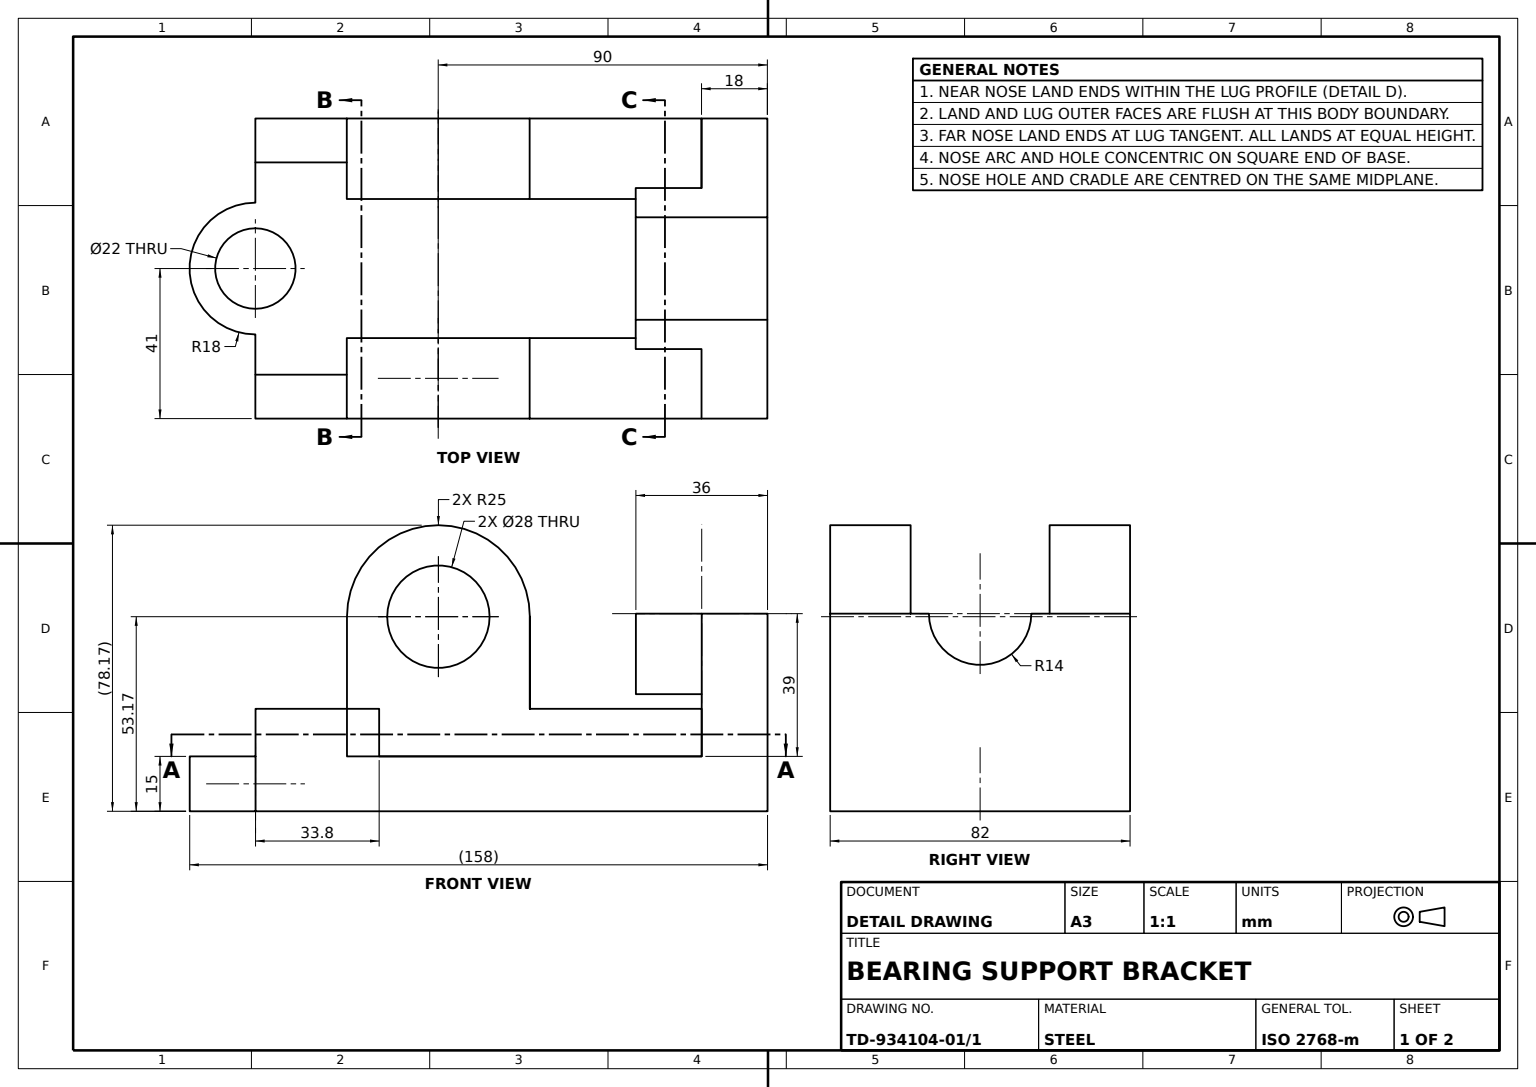
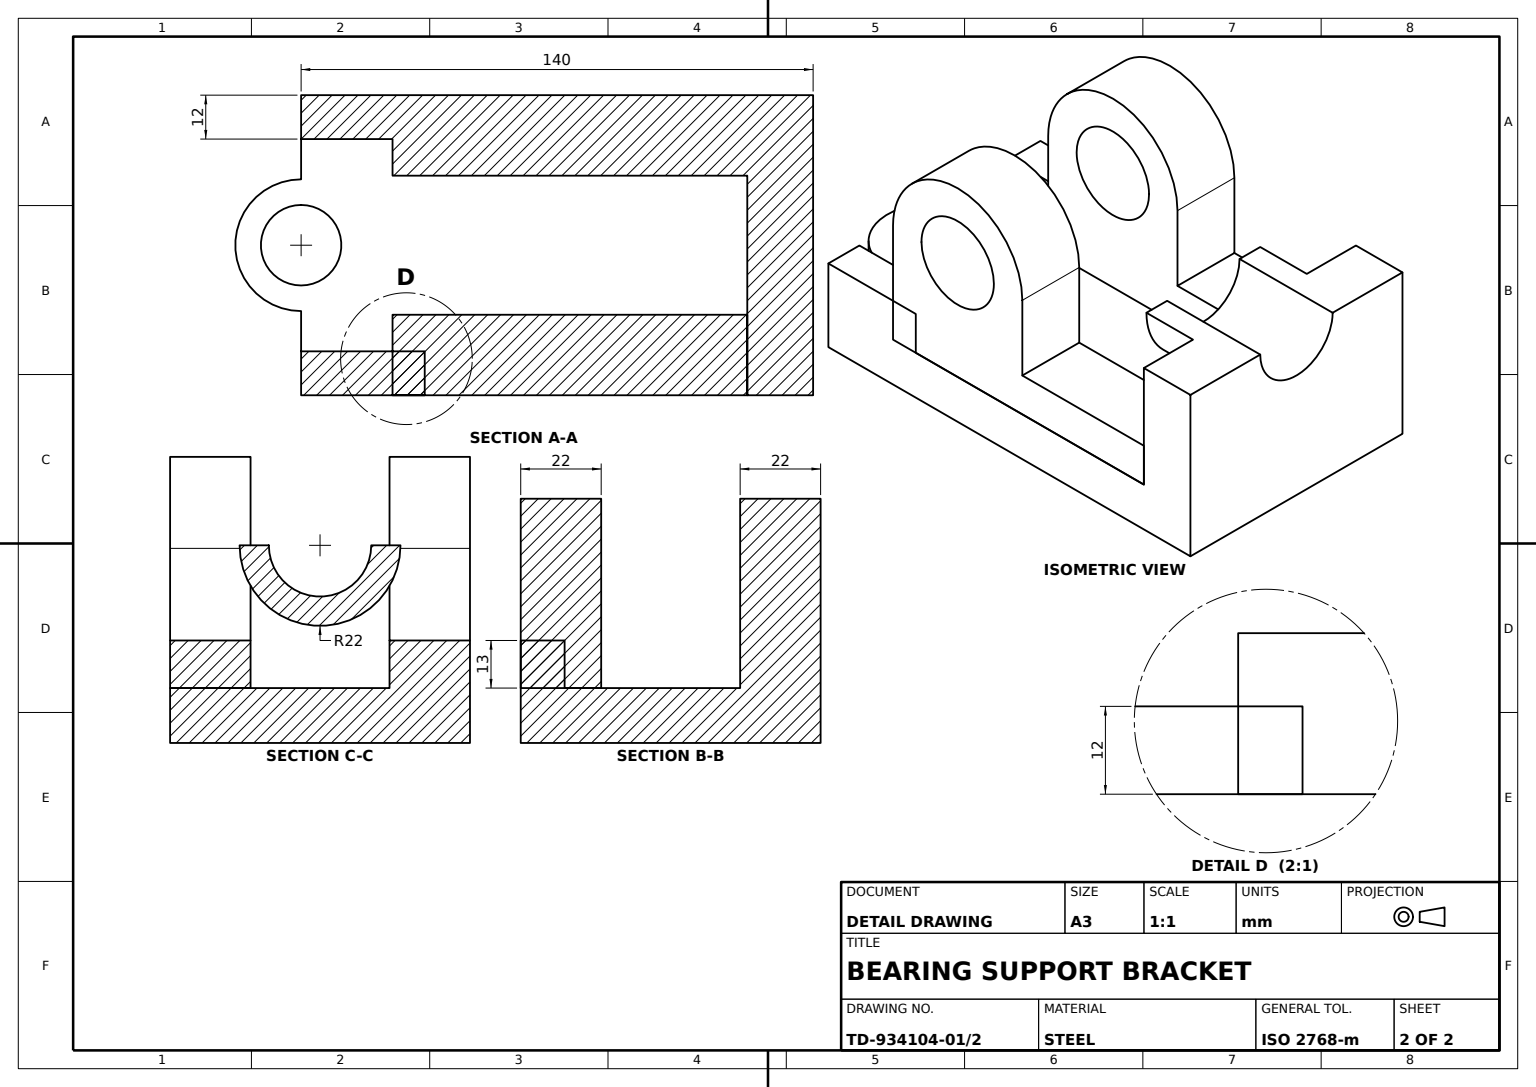
from build123d import *

# Parameters (mm, degrees)
BASE_PLATE_SKETCH_W        = 140
BASE_PLATE_SKETCH_H        = 82
BASE_PLATE_140X82X15_DEPTH = 7.5
SIDE_WALL_SKETCH_W         = 18
SIDE_WALL_SKETCH_H         = 82
SIDE_WALL_DEPTH            = 39
WALL_EXTENSION_DEPTH       = 18
WALL_SLOT_CUT_DEPTH        = 18
END_BLOCK_DEPTH            = 13
BEARING_LUG_DEPTH          = 22
LUG_BORE_DEPTH             = 129.91094718
LUG_BORE_DEPTH_BACK        = 129.91094718
LUG_BORE_SKETCH_R          = 14
CRADLE_BOSS_SKETCH_R       = 18
CRADLE_BOSS_DEPTH          = 15
CRADLE_SKETCH_R            = 11
CRADLE_CUT_DEPTH           = 15


with BuildPart() as part:
    # Base Plate Sketch → Base Plate 140x82x15 (new, symmetric)
    with BuildSketch(Plane(origin=(0, 0, 0), x_dir=(1, 0, 0), z_dir=(0, 1, 0))):
        Rectangle(BASE_PLATE_SKETCH_W, BASE_PLATE_SKETCH_H)
    extrude(amount=BASE_PLATE_140X82X15_DEPTH, both=True)

    # Side Wall Sketch → Side Wall (add)
    with BuildSketch(Plane(origin=(0, 7.5, 0), x_dir=(1, 0, 0), z_dir=(0, 1, 0))):
        with Locations((61, 0)):
            Rectangle(SIDE_WALL_SKETCH_W, SIDE_WALL_SKETCH_H)
    extrude(amount=SIDE_WALL_DEPTH)

    # Wall Extension Sketch → Wall Extension (add)
    with BuildSketch(Plane.ZY.offset(-52)):
        with BuildLine():
            Line((-14, 46.5), (-22, 46.5))
            ThreePointArc((-22, 46.5), (0, 24.5), (22, 46.5))
            Line((22, 46.5), (14, 46.5))
            ThreePointArc((14, 46.5), (0, 32.5), (-14, 46.5))
        make_face()
    extrude(amount=WALL_EXTENSION_DEPTH)

    # Wall Slot Sketch → Wall Slot Cut (cut)
    with BuildSketch(Plane(origin=(70, 0, 0), x_dir=(0, 0, -1), z_dir=(1, 0, 0))):
        with BuildLine():
            Line((-14, 46.5), (14, 46.5))
            ThreePointArc((14, 46.5), (0, 32.5), (-14, 46.5))
        make_face()
    extrude(amount=-WALL_SLOT_CUT_DEPTH, mode=Mode.SUBTRACT)

    # End Block Sketch → End Block (add)
    with BuildSketch(Plane(origin=(0, 7.5, 0), x_dir=(1, 0, 0), z_dir=(0, 1, 0))):
        Polygon((-70, -38.536273507), (-70, -41), (-36.2, -41), (-36.2, -29), (-70, -29), (-70, -37.053252514), align=None)
    end_block = extrude(amount=END_BLOCK_DEPTH)


with BuildPart() as body_2:
    # Bearing Lug Sketch → Bearing Lug (new body)
    with BuildSketch(Plane.XY.offset(41)):
        with BuildLine():
            Line((-45, 45.668467528), (-45, 7.5))
            Line((-45, 7.5), (52, 7.5))
            Line((52, 7.5), (52, 20.5))
            Line((52, 20.5), (5, 20.5))
            Line((5, 20.5), (5, 45.668467528))
            ThreePointArc((5, 45.668467528), (-20, 70.668467528), (-45, 45.668467528))
        make_face()
    bearing_lug = extrude(amount=-BEARING_LUG_DEPTH)


with BuildPart() as part_1:
    add(part.part)

    # Bearing Lug Mirror: Bearing Lug across plane
    add(bearing_lug.mirror(Plane.XY))

    # End Block Mirror: End Block across plane
    add(end_block.mirror(Plane.XY))


with BuildPart() as lug_bore_tool:
    # Lug Bore Sketch → Lug Bore (new, two sides: drawn at the far end of the back side and taken through both)
    with BuildSketch(Plane.XY.offset(41).offset(-LUG_BORE_DEPTH_BACK)):
        with Locations((-20, 45.668467528)):
            Circle(LUG_BORE_SKETCH_R)
    extrude(amount=LUG_BORE_DEPTH + LUG_BORE_DEPTH_BACK)


with BuildPart() as part_2:
    add(part_1.part)

    # Lug Bore: cut by lug_bore_tool
    add(lug_bore_tool.part, mode=Mode.SUBTRACT)

    # Cradle Boss Sketch → Cradle Boss (add)
    with BuildSketch(Plane(origin=(0, 7.5, 0), x_dir=(1, 0, 0), z_dir=(0, 1, 0))):
        with Locations((-70, 0)):
            Circle(CRADLE_BOSS_SKETCH_R)
    extrude(amount=-CRADLE_BOSS_DEPTH)

    # Cradle Sketch → Cradle Cut (cut)
    with BuildSketch(Plane(origin=(0, 7.5, 0), x_dir=(1, 0, 0), z_dir=(0, 1, 0))):
        with Locations(Location((-70, 0, 0), (0, 0, 270))):
            Circle(CRADLE_SKETCH_R)
    extrude(amount=-CRADLE_CUT_DEPTH, mode=Mode.SUBTRACT)


with BuildPart() as body_2_1:
    add(body_2.part)

    # Lug Bore: cut by lug_bore_tool
    add(lug_bore_tool.part, mode=Mode.SUBTRACT)


solid = Compound([part_2.part, body_2_1.part])
